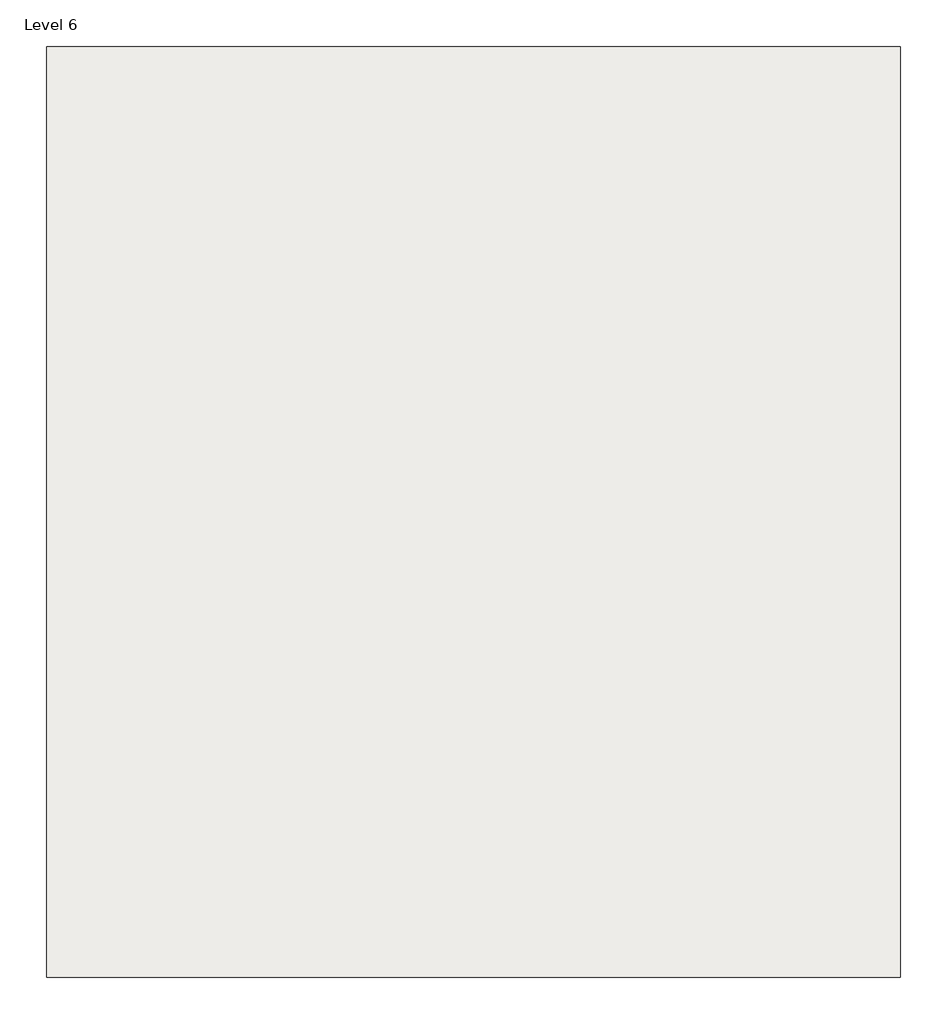
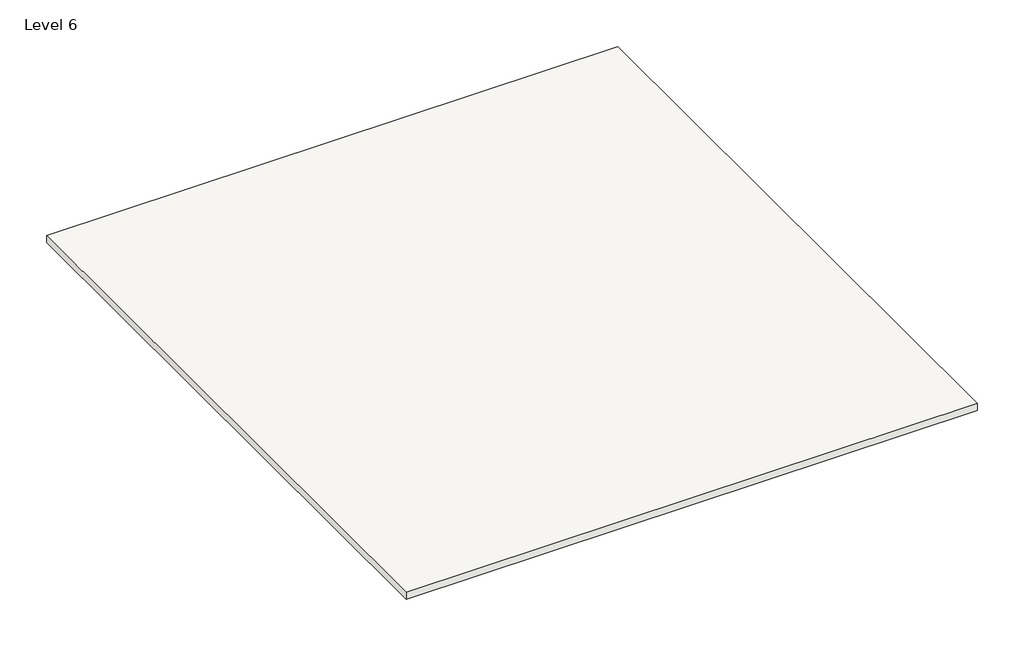
# One storey, incomplete: 1 roof.
"""IFC4 building model written with IfcOpenShell, lengths in millimetres."""

from ifc_helpers import new_model, si_unit, frame, origin, place, context, project, spatial, polyline, outline, extrude, element, save

model = new_model("IFC4")

# Units and contexts
model_context = context("Model", 3, world=origin())
ifc_project = project(units=[si_unit("LENGTHUNIT", "METRE", prefix="MILLI")], contexts=[model_context])

# Site, building, storey
site = spatial("IfcSite", under=ifc_project)
building = spatial("IfcBuilding", under=site)
storey = spatial("IfcBuildingStorey", under=building, Name="Level 6", Elevation=12801.6)

# Roof
placement = place(None, origin())
element("IfcRoof", 1, ObjectType="Generic - 12\"", at=placement, inside=storey, context=model_context, shape_type="SweptSolid", body=[
    extrude(outline(polyline([(-7252.5317864, 7748.8034997), (4771.8282136, 7748.8034997), (4771.8282136, -5357.5965003), (-7252.5317864, -5357.5965003), (-7252.5317864, 7748.8034997)])), frame((0.0, 0.0, 12649.2), z_axis=(0.0, 0.0, 1.0), x_axis=(1.0, 0.0, 0.0)), (0.0, 0.0, 1.0), 152.4),
])

save(model, "model.ifc")

# Revit data of these elements
# Type "Generic - 12\""
#   Assembly Code = "B1020"
#   Layers, outside or top first: 0' - 6" no material (function 1)
# Element 1 (IfcRoof, "Generic - 12\"")
#   built-in parameter 1001705 = 42 (stored number, unit not read)
#   built-in parameter 1001701 = -0.5 (stored number, unit not read)
#   built-in parameter 1001710 = 33615
#   Phase Created = New Construction
#   Materials on its faces: "Default Roof"
# Materials
#   "Default Roof": colour RGB 88 101 114, transparency 0, Cost = 0
